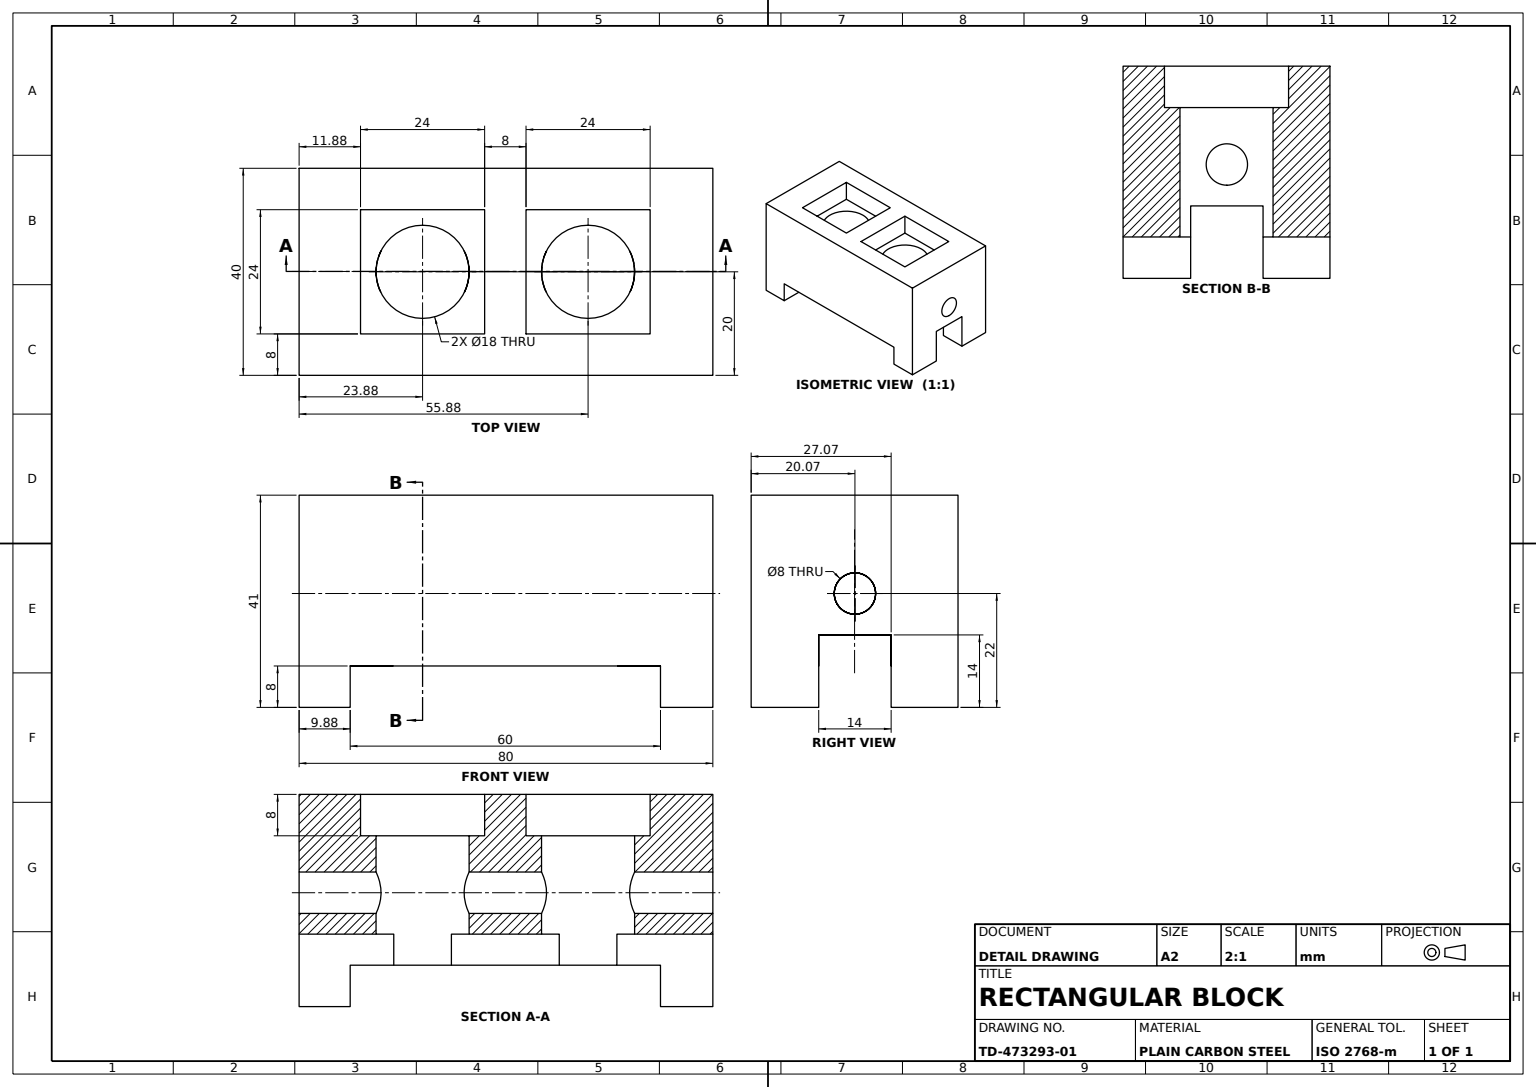
from build123d import *

# Parameters (mm, degrees)
BASE_BLOCK_40_DEPTH          = 40
SQUARE_POCKETS_SKETCH_W      = 24
SQUARE_POCKETS_SKETCH_H      = 24
SQUARE_POCKETS_2X24X24_DEPTH = 8
POCKET_HOLES_SKETCH_R        = 9
POCKET_HOLES_2X_12_DEPTH     = 66.566879024
END_BORE_AND_SLOT_SKETCH_R   = 4
END_BORE_AND_SLOT_SKETCH_W   = 14
END_BORE_AND_SLOT_SKETCH_H   = 14
END_BORE_AND_SLOT_DEPTH      = 96.336247042


with BuildPart() as part:
    # Block Profile Sketch → Base Block 40 (new body)
    with BuildSketch(Plane.XY):
        Polygon((-30, 0), (30, 0), (30, -8), (40.125, -8), (40.125, 33), (-39.875, 33), (-39.875, -8), (-30, -8), align=None)
    extrude(amount=-BASE_BLOCK_40_DEPTH)

    # Square Pockets Sketch → Square Pockets 2x24x24 (cut)
    with BuildSketch(Plane(origin=(0, 33, 0), x_dir=(1, 0, 0), z_dir=(0, 1, 0))):
        with Locations((-16, 20)):
            Rectangle(SQUARE_POCKETS_SKETCH_W, SQUARE_POCKETS_SKETCH_H)
        with Locations((16, 20)):
            Rectangle(SQUARE_POCKETS_SKETCH_W, SQUARE_POCKETS_SKETCH_H)
    extrude(amount=-SQUARE_POCKETS_2X24X24_DEPTH, mode=Mode.SUBTRACT)

    # Pocket Holes Sketch → Pocket Holes 2xØ12 (cut, through all)
    with BuildSketch(Plane(origin=(0, 25, 0), x_dir=(1, 0, 0), z_dir=(0, 1, 0))):
        with Locations(Location((-16, 20, 0), (0, 0, 270))):
            Circle(POCKET_HOLES_SKETCH_R)
        with Locations(Location((16, 20, 0), (0, 0, 90))):
            Circle(POCKET_HOLES_SKETCH_R)
    extrude(amount=-POCKET_HOLES_2X_12_DEPTH, mode=Mode.SUBTRACT)

    # End Bore and Slot Sketch → End Bore and Slot (cut, through all)
    with BuildSketch(Plane(origin=(40.125, 0, 0), x_dir=(0, 0, -1), z_dir=(1, 0, 0))):
        with Locations(Location((20.067495301, 14, 0), (0, 0, 90))):
            Circle(END_BORE_AND_SLOT_SKETCH_R)
        with Locations((20.067495301, -1)):
            Rectangle(END_BORE_AND_SLOT_SKETCH_W, END_BORE_AND_SLOT_SKETCH_H)
    extrude(amount=-END_BORE_AND_SLOT_DEPTH, mode=Mode.SUBTRACT)


solid = part.part
